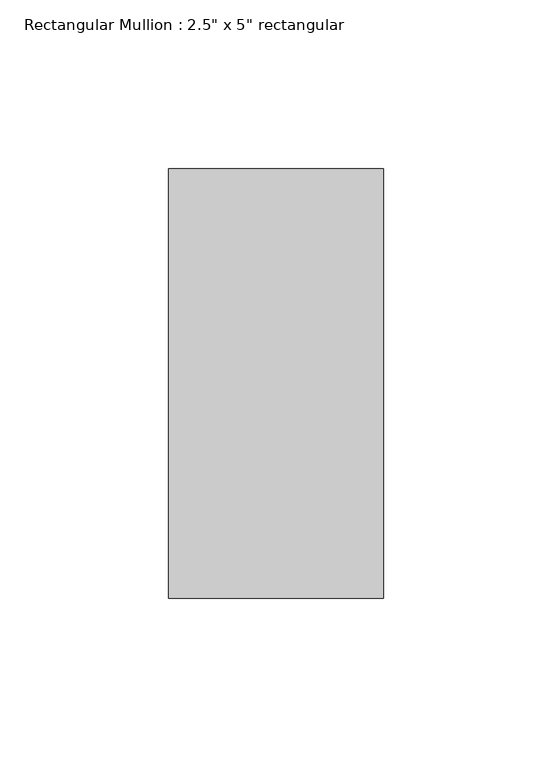
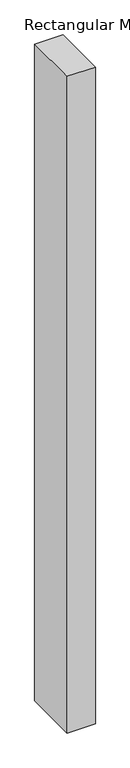
"""IFC4 building model written with IfcOpenShell, lengths in millimetres: member geometry."""

from ifc_helpers import new_model, si_unit, frame, origin, place, context, project, spatial, polyline, outline, extrude, source, transform, mapped, element, save


def member_39095dcb(model_context):
    return source(origin(), model_context, "Body", "SweptSolid", [
        extrude(outline(polyline([(31.75, 63.5), (31.75, -63.5), (-31.75, -63.5), (-31.75, 63.5), (31.75, 63.5)])), frame((0.0, 0.0, -1566.9800364), z_axis=(0.0, 0.0, 1.0), x_axis=(1.0, 0.0, 0.0)), (0.0, 0.0, 1.0), 1566.9800364),
    ])


if __name__ == "__main__":
    model = new_model("IFC4")
    model_context = context("Model", 3, world=origin())
    ifc_project = project(units=[si_unit("LENGTHUNIT", "METRE", prefix="MILLI")], contexts=[model_context])
    site = spatial("IfcSite", under=ifc_project)
    building = spatial("IfcBuilding", under=site)
    placement = place(None, origin())
    member_shape = member_39095dcb(model_context)
    element("IfcMember", 1, ObjectType="Rectangular Mullion : 2.5\" x 5\" rectangular", at=placement, inside=building, context=model_context, shape_type="MappedRepresentation", body=[
        mapped(member_shape, transform((0.0, 0.0, 0.0), x_axis=(1.0, 0.0, 0.0), y_axis=(0.0, 1.0, 0.0), z_axis=(0.0, 0.0, 1.0))),
    ])
    save(model, "model.ifc")

# Revit data of these elements
# Type "Rectangular Mullion : 2.5\" x 5\" rectangular"
#   built-in parameter 1007304 = 0.416667 (stored number, unit not read)
#   built-in parameter 1007301 = 0.104167 (stored number, unit not read)
#   built-in parameter 1007300 = 0.104167 (stored number, unit not read)
# Element 1 (IfcMember, "Rectangular Mullion : 2.5\" x 5\" rectangular")
#   Materials on its faces: "Aluminum"
# Materials
#   "Aluminum": class "Metal", colour RGB 247 247 247, transparency 0, Description = "Aluminum 6061", Cost = 0
